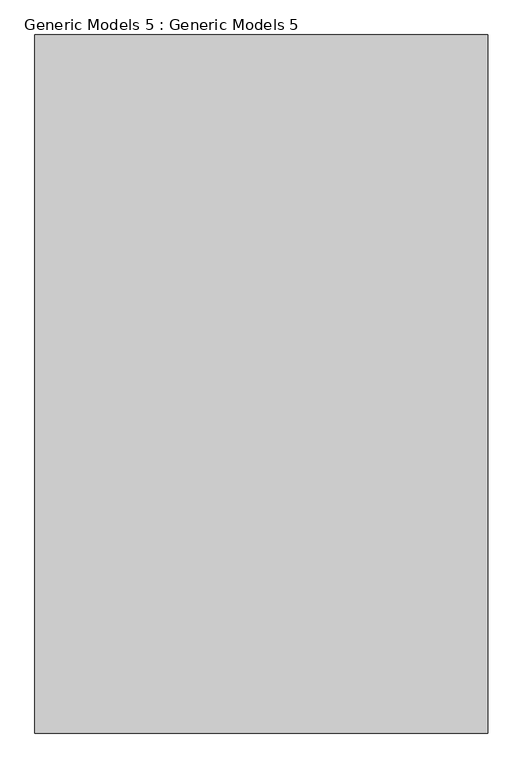
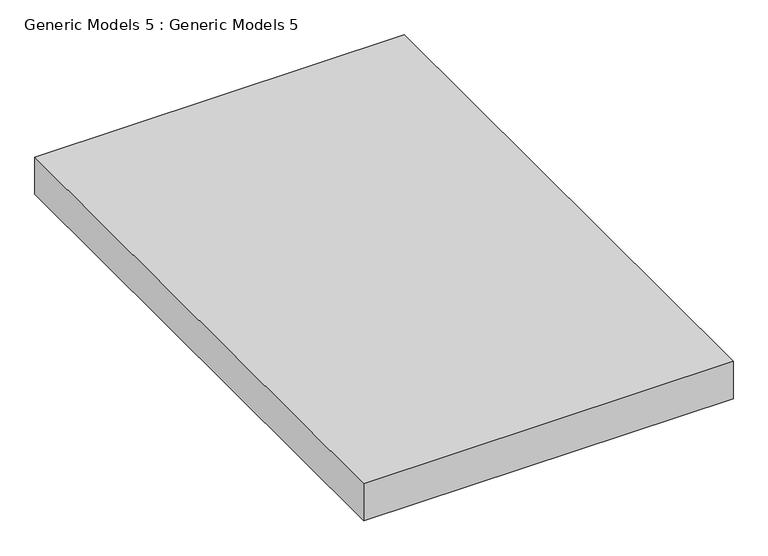
"""IFC4 building model written with IfcOpenShell, lengths in millimetres: proxy geometry, Generic Models 5 : Generic Models 5."""

from ifc_helpers import new_model, si_unit, frame, origin, place, context, project, spatial, polyline, outline, extrude, source, transform, mapped, element, save


def generic_models_5_generic_models_5_8773877a(model_context):
    return source(origin(), model_context, "Body", "SweptSolid", [
        extrude(outline(polyline([(1011.5606661, -4090.1262081), (-1732.8511383, -4090.1262081), (-1732.8511383, 139.1133697), (1011.5606661, 139.1133697), (1011.5606661, -4090.1262081)])), frame((0.0, 0.0, 6108.9199799), z_axis=(0.0, 0.0, 1.0), x_axis=(1.0, 0.0, 0.0)), (0.0, 0.0, 1.0), 291.8800201),
    ])


if __name__ == "__main__":
    model = new_model("IFC4")
    model_context = context("Model", 3, world=origin())
    ifc_project = project(units=[si_unit("LENGTHUNIT", "METRE", prefix="MILLI")], contexts=[model_context])
    site = spatial("IfcSite", under=ifc_project)
    building = spatial("IfcBuilding", under=site)
    placement = place(None, origin())
    generic_models_5_generic_models_5_shape = generic_models_5_generic_models_5_8773877a(model_context)
    element("IfcBuildingElementProxy", 1, Name="Generic Models 5 : Generic Models 5", ObjectType="Generic Models 5 : Generic Models 5", at=placement, inside=building, context=model_context, shape_type="MappedRepresentation", body=[
        mapped(generic_models_5_generic_models_5_shape, transform((0.0, 0.0, 0.0), x_axis=(1.0, 0.0, 0.0), y_axis=(0.0, 1.0, 0.0), z_axis=(0.0, 0.0, 1.0))),
    ])
    save(model, "model.ifc")

# Revit data of these elements
# Element 1 (IfcBuildingElementProxy, "Generic Models 5 : Generic Models 5")
#   Materials on its faces: "Clad - White"
# Materials
#   "Clad - White": class "Wood", colour RGB 242 242 238, transparency 0, Cost = 0
